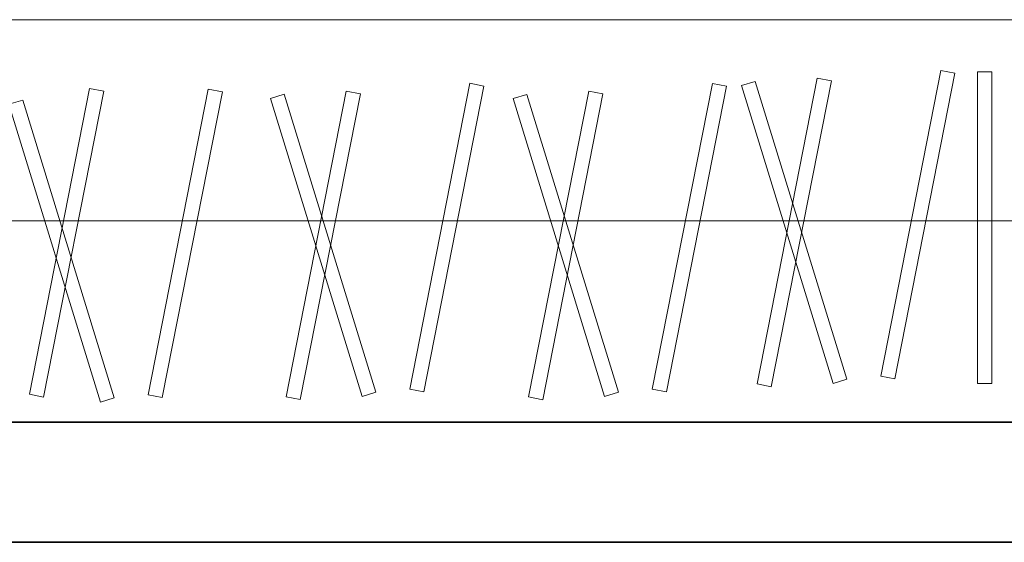
# Model space of a CAD drawing. Units: inches. Extents: x -61 to 1599, y -1316 to 257.
# Tile 179 of 204: x 1395 to 1444, y -783 to -757. Entities that reach past the tile are written whole.
import ezdxf

# ---------------------------------------------------------------- set-up
doc = ezdxf.new("R2010")
doc.units = ezdxf.units.IN
doc.header["$MEASUREMENT"] = 0
doc.layers.add('A-FLOR-CASE', color=8, linetype='Continuous', lineweight=18)
doc.layers.add('WALLS', color=4, linetype='Continuous', lineweight=35)

# ---------------------------------------------------------------- blocks, each defined once
blk = doc.blocks.new('WARDROBE-HANGING')
blk.add_line((10.047, 0), (10.047, 68))
for points in [[(20.094, 0), (0, 0), (0, 68), (20.094, 68)], [(2.482, 67.852), (17.751, 64.849), (17.612, 64.142), (2.343, 67.146)], [(1.346, 59.162), (16.221, 63.731), (16.432, 63.043), (1.557, 58.474)], [(1.325, 62.957), (16.593, 59.954), (16.454, 59.247), (1.186, 62.251)], [(1.713, 56.784), (16.981, 53.781), (16.842, 53.074), (1.574, 56.078)], [(0.997, 46.467), (15.872, 51.036), (16.084, 50.348), (1.209, 45.779)], [(1.394, 50.014), (16.662, 47.011), (16.523, 46.305), (1.255, 49.308)], [(1.365, 44.09), (16.633, 41.086), (16.494, 40.38), (1.226, 43.383)], [(1.283, 33.408), (16.158, 37.977), (16.37, 37.289), (1.495, 32.72)], [(1.262, 37.203), (16.53, 34.2), (16.391, 33.493), (1.123, 36.497)], [(1.651, 31.03), (16.919, 28.027), (16.78, 27.32), (1.512, 30.324)], [(1.279, 21.299), (16.154, 25.868), (16.365, 25.18), (1.49, 20.611)], [(1.257, 25.094), (16.525, 22.091), (16.386, 21.384), (1.118, 24.388)], [(1.646, 18.921), (16.914, 15.918), (16.775, 15.211), (1.507, 18.215)], [(1.928, 9.892), (16.803, 14.461), (17.014, 13.773), (2.139, 9.203)], [(1.906, 13.687), (17.174, 10.684), (17.035, 9.977), (1.767, 12.981)], [(2.295, 7.514), (17.563, 4.511), (17.424, 3.804), (2.156, 6.808)], [(17.491, 1.962), (1.93, 1.962), (1.93, 2.682), (17.491, 2.682)]]:
    blk.add_lwpolyline(points, close=True)

msp = doc.modelspace()

# ---------------------------------------------------------------- linework, layer by layer
at = {"layer": 'WALLS'}
for p, q in [((1375.7028, -777.169), (1513.7028, -777.169)), ((1375.7028, -783.169), (1513.7028, -783.169))]:
    msp.add_line(p, q, dxfattribs=at)

# ---------------------------------------------------------------- block references
at = {"layer": 'A-FLOR-CASE', "rotation": 90.00000000000018}
msp.add_blockref('WARDROBE-HANGING', (1445.7029, -777.1692), dxfattribs=at)

doc.saveas('drawing.dxf')
